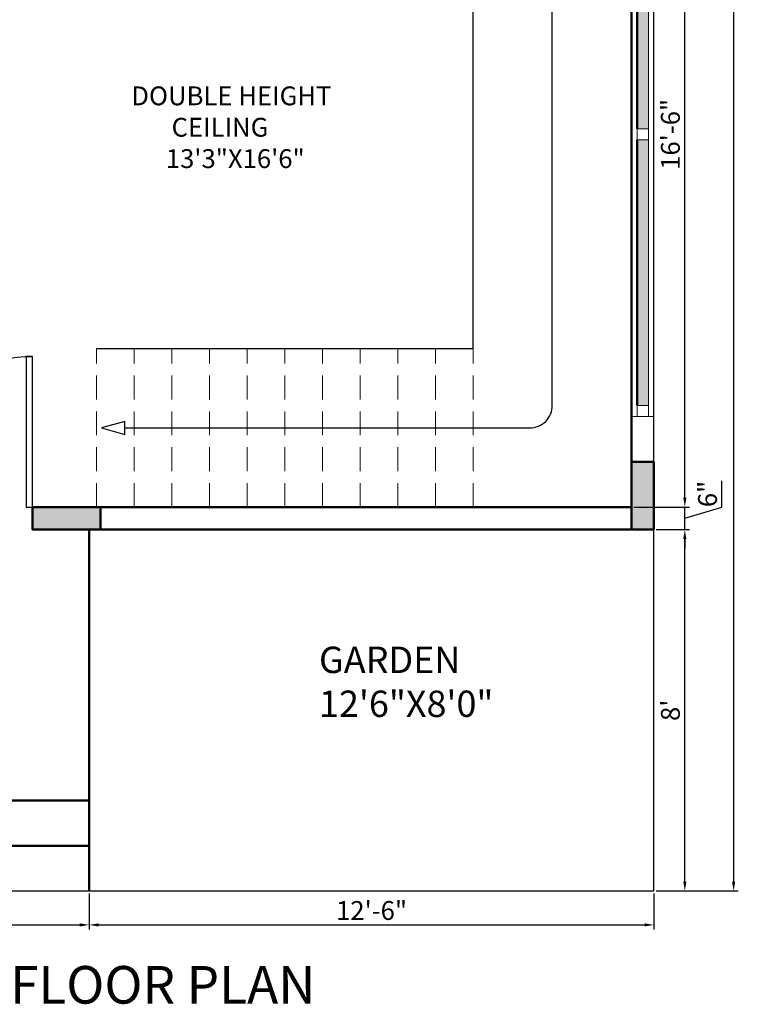
# Model space of a CAD drawing. Units: inches. Extents: x 3064 to 19385, y 846 to 15425.
# Tile 27 of 108: x 4938 to 5129, y 846 to 1108. Entities that reach past the tile are written whole.
import ezdxf

# ---------------------------------------------------------------- set-up
doc = ezdxf.new("R2010")
doc.units = ezdxf.units.IN
doc.linetypes.add('DASHED', pattern=[19.05, 12.7, -6.35])
for name, color, linetype, lineweight in [('A-ANNO-DIMS', 2, 'Continuous', 18), ('A-ANNO-TEXT', 7, 'Continuous', 25), ('A-AREA-IDEN', 3, 'Continuous', 18), ('A-COLS', 1, 'Continuous', 35), ('A-DOOR', 3, 'Continuous', 25), ('A-FLOR-STRS', 2, 'Continuous', 25), ('A-FLOR-STRS-OVHD', 2, 'DASHED', 18), ('A-GLAZ', 4, 'Continuous', 18), ('A-WALL', 7, 'Continuous', 50), ('C-PROP', 6, 'Continuous', 25)]:
    doc.layers.add(name, color=color, linetype=linetype, lineweight=lineweight)
doc.styles.get("Standard").update_dxf_attribs({"font": 'arial.ttf'})
doc.dimstyles.new('ISO-25', dxfattribs={"dimtxt": 9, "dimasz": 2.5, "dimexe": 1.25, "dimexo": 0.625, "dimtad": 1, "dimdec": 1, "dimlunit": 3, "dimtxsty": 'Standard', "dimcen": 2.5, "dimadec": 0, "dimazin": 0, "dimtfac": 1, "dimtdec": 1, "dimtmove": 0, "dimatfit": 3, "dimfxl": 1, "dimarcsym": 0})

# ---------------------------------------------------------------- blocks, each defined once
blk = doc.blocks.new('*U2')
for p, q in [((0, 0), (0, -6)), ((40, 0), (40, -6))]:
    blk.add_line(p, q)
blk.add_lwpolyline([(0, 0), (0, 40), (1.75, 40), (1.75, 0)], close=True)
blk.add_arc((0, 0), 40, 0, 90)
blk = doc.blocks.new('*D56')
at = {"layer": 'A-ANNO-DIMS', "color": 0, "lineweight": -2, "transparency": 16777216}
for p, q in [((4764.48, 875.47), (4764.48, 865.83)), ((4956.48, 875.47), (4956.48, 865.83)), ((4766.98, 867.08), (4953.98, 867.08))]:
    blk.add_line(p, q, dxfattribs=at)
at = {"layer": 'A-ANNO-DIMS', "color": 0, "transparency": 16777216}
for points in [[(4766.98, 867.5), (4766.98, 866.67), (4764.48, 867.08)], [(4953.98, 867.5), (4953.98, 866.67), (4956.48, 867.08)]]:
    blk.add_solid(points, dxfattribs=at)
at = {"layer": 'Defpoints', "color": 0, "transparency": 16777216}
for p in [(4764.48, 876.1), (4956.48, 876.1), (4956.48, 867.08)]:
    blk.add_point(p, dxfattribs=at)
at = {"layer": 'A-ANNO-DIMS', "color": 0, "transparency": 16777216, "insert": (4860.48, 870.26), "char_height": 5, "attachment_point": 5}
blk.add_mtext("16'", dxfattribs=at)
blk = doc.blocks.new('*D57')
at = {"layer": 'A-ANNO-DIMS', "color": 0, "lineweight": -2, "transparency": 16777216}
for p, q in [((4956.48, 875.47), (4956.48, 865.83)), ((5106.48, 875.47), (5106.48, 865.83)), ((4958.98, 867.08), (5103.98, 867.08))]:
    blk.add_line(p, q, dxfattribs=at)
at = {"layer": 'A-ANNO-DIMS', "color": 0, "transparency": 16777216}
for points in [[(4958.98, 867.5), (4958.98, 866.67), (4956.48, 867.08)], [(5103.98, 867.5), (5103.98, 866.67), (5106.48, 867.08)]]:
    blk.add_solid(points, dxfattribs=at)
at = {"layer": 'Defpoints', "color": 0, "transparency": 16777216}
for p in [(4956.48, 876.1), (5106.48, 876.1), (5106.48, 867.08)]:
    blk.add_point(p, dxfattribs=at)
at = {"layer": 'A-ANNO-DIMS', "color": 0, "transparency": 16777216, "insert": (5031.48, 870.26), "char_height": 5, "attachment_point": 5}
blk.add_mtext('12\'-6"', dxfattribs=at)
blk = doc.blocks.new('*D58')
at = {"layer": 'A-ANNO-DIMS', "color": 0, "lineweight": -2, "transparency": 16777216}
for p, q in [((5107.1, 972.1), (5115.92, 972.1)), ((5114.67, 878.6), (5114.67, 969.6)), ((5107.1, 876.1), (5115.92, 876.1))]:
    blk.add_line(p, q, dxfattribs=at)
at = {"layer": 'A-ANNO-DIMS', "color": 0, "transparency": 16777216}
for points in [[(5114.25, 969.6), (5115.09, 969.6), (5114.67, 972.1)], [(5114.25, 878.6), (5115.09, 878.6), (5114.67, 876.1)]]:
    blk.add_solid(points, dxfattribs=at)
at = {"layer": 'Defpoints', "color": 0, "transparency": 16777216}
for p in [(5106.48, 972.1), (5114.67, 972.1), (5106.48, 876.1)]:
    blk.add_point(p, dxfattribs=at)
at = {"layer": 'A-ANNO-DIMS', "color": 0, "transparency": 16777216, "insert": (5111.49, 924.1), "char_height": 5, "attachment_point": 5, "rotation": 90}
blk.add_mtext("8'", dxfattribs=at)
blk = doc.blocks.new('*D59')
at = {"layer": 'A-ANNO-DIMS', "color": 0, "lineweight": -2, "transparency": 16777216}
for p, q in [((5124.52, 978.05), (5124.52, 985.07)), ((5114.67, 980.6), (5114.67, 983.1)), ((5101.1, 978.1), (5115.92, 978.1)), ((5114.67, 972.1), (5114.67, 978.1)), ((5114.67, 972.1), (5114.67, 978.1)), ((5114.67, 975.1), (5124.52, 978.05)), ((5107.1, 972.1), (5115.92, 972.1)), ((5114.67, 969.6), (5114.67, 967.1))]:
    blk.add_line(p, q, dxfattribs=at)
at = {"layer": 'A-ANNO-DIMS', "color": 0, "transparency": 16777216}
for points in [[(5114.25, 980.6), (5115.09, 980.6), (5114.67, 978.1)], [(5114.25, 969.6), (5115.09, 969.6), (5114.67, 972.1)]]:
    blk.add_solid(points, dxfattribs=at)
at = {"layer": 'Defpoints', "color": 0, "transparency": 16777216}
for p in [(5100.48, 978.1), (5114.67, 978.1), (5106.48, 972.1)]:
    blk.add_point(p, dxfattribs=at)
at = {"layer": 'A-ANNO-DIMS', "color": 0, "transparency": 16777216, "insert": (5121.34, 981.56), "char_height": 5, "attachment_point": 5, "rotation": 90}
blk.add_mtext('6"', dxfattribs=at)
blk = doc.blocks.new('*D60')
at = {"layer": 'A-ANNO-DIMS', "color": 0, "lineweight": -2, "transparency": 16777216}
for p, q in [((5101.1, 1176.1), (5115.92, 1176.1)), ((5114.67, 980.6), (5114.67, 1173.6)), ((5101.1, 978.1), (5115.92, 978.1))]:
    blk.add_line(p, q, dxfattribs=at)
at = {"layer": 'A-ANNO-DIMS', "color": 0, "transparency": 16777216}
for points in [[(5114.25, 1173.6), (5115.09, 1173.6), (5114.67, 1176.1)], [(5114.25, 980.6), (5115.09, 980.6), (5114.67, 978.1)]]:
    blk.add_solid(points, dxfattribs=at)
at = {"layer": 'Defpoints', "color": 0, "transparency": 16777216}
for p in [(5100.48, 1176.1), (5114.67, 1176.1), (5100.48, 978.1)]:
    blk.add_point(p, dxfattribs=at)
at = {"layer": 'A-ANNO-DIMS', "color": 0, "transparency": 16777216, "insert": (5111.49, 1077.1), "char_height": 5, "attachment_point": 5, "rotation": 90}
blk.add_mtext('16\'-6"', dxfattribs=at)
blk = doc.blocks.new('*D66')
at = {"layer": 'A-ANNO-DIMS', "color": 0, "lineweight": -2, "transparency": 16777216}
for p, q in [((5107.1, 1392.1), (5128.87, 1392.1)), ((5127.62, 1389.6), (5127.62, 878.6)), ((5107.1, 876.1), (5128.87, 876.1))]:
    blk.add_line(p, q, dxfattribs=at)
at = {"layer": 'A-ANNO-DIMS', "color": 0, "transparency": 16777216}
for points in [[(5127.2, 1389.6), (5128.04, 1389.6), (5127.62, 1392.1)], [(5127.2, 878.6), (5128.04, 878.6), (5127.62, 876.1)]]:
    blk.add_solid(points, dxfattribs=at)
at = {"layer": 'Defpoints', "color": 0, "transparency": 16777216}
for p in [(5106.48, 1392.1), (5106.48, 876.1), (5127.62, 876.1)]:
    blk.add_point(p, dxfattribs=at)
at = {"layer": 'A-ANNO-DIMS', "color": 0, "transparency": 16777216, "insert": (5124.44, 1134.1), "char_height": 5, "attachment_point": 5, "rotation": 90}
blk.add_mtext("43'", dxfattribs=at)
blk = doc.blocks.new('WIN-1800-PAIR')
h = blk.add_hatch(color=256)
h.dxf.hatch_style = 1
h.paths.add_polyline_path([(0, 0), (3, 0), (3, 70.5), (0, 70.5)])
h.paths.add_polyline_path([(3, 144), (0, 144), (0, 73.5), (3, 73.5)])
blk.add_line((3, 144), (3, 73.5))
blk.add_lwpolyline([(3, 144), (0, 144), (0, 147), (3, 147)], close=True)
blk = doc.blocks.new('WIN-2000')
blk.add_line((3, 0), (3, 70.5))
blk.add_lwpolyline([(3, 70.5), (0, 70.5), (0, 73.5), (3, 73.5)], close=True)

msp = doc.modelspace()

# ---------------------------------------------------------------- hatches: boundary and pattern name
at = {"layer": 'A-COLS'}
h = msp.add_hatch(color=256, dxfattribs=at)
h.dxf.hatch_style = 1
h.paths.add_polyline_path([(5106.48, 972.1), (5106.48, 990.1), (5100.48, 990.1), (5100.48, 972.1)])
h = msp.add_hatch(color=256, dxfattribs=at)
h.dxf.hatch_style = 1
h.paths.add_polyline_path([(4959.48, 978.1), (4941.48, 978.1), (4941.48, 972.1), (4959.48, 972.1)])

# ---------------------------------------------------------------- linework, layer by layer
at = {"layer": 'A-FLOR-STRS'}
for q in [(5058.48, 1176.1), (4958.48, 1020.1)]:
    msp.add_line((5058.48, 1020.1), q, dxfattribs=at)
msp.add_lwpolyline([(4965.97, 999.1), (5073.48, 999.1, 0.414214), (5079.48, 1005.1), (5079.48, 1149.1, 0.414214), (5073.48, 1155.1), (4946.48, 1155.1)], format="xyb", dxfattribs=at)
msp.add_lwpolyline([(4959.77, 999.1), (4965.97, 997.36), (4965.97, 1000.83)], close=True, dxfattribs=at)
at = {"layer": 'A-FLOR-STRS-OVHD', "ltscale": 0.5}
for p, q in [((4958.48, 978.1), (4958.48, 1020.1)), ((4968.48, 978.1), (4968.48, 1020.1)), ((4978.48, 978.1), (4978.48, 1020.1)), ((4988.48, 978.1), (4988.48, 1020.1)), ((4998.48, 978.1), (4998.48, 1020.1)), ((5008.48, 978.1), (5008.48, 1020.1)), ((5018.48, 978.1), (5018.48, 1020.1)), ((5028.48, 978.1), (5028.48, 1020.1)), ((5038.48, 978.1), (5038.48, 1020.1)), ((5048.48, 978.1), (5048.48, 1020.1)), ((5058.48, 978.1), (5058.48, 1020.1))]:
    msp.add_line(p, q, dxfattribs=at)
at = {"layer": 'A-GLAZ'}
msp.add_line((5106.48, 1002.1), (5100.48, 1002.1), dxfattribs=at)
msp.add_line((5106.48, 1002.1), (5100.48, 1002.1), dxfattribs=at)
msp.add_lwpolyline([(5104.98, 1002.1), (5101.98, 1002.1), (5101.98, 1005.1), (5104.98, 1005.1)], close=True, dxfattribs=at)
at = {"layer": 'A-WALL'}
for p, q in [((5100.48, 978.1), (5100.48, 1176.1)), ((5101.98, 1149.1), (5101.98, 1078.6)), ((5101.98, 1005.1), (5101.98, 1075.6)), ((5100.48, 978.1), (4941.48, 978.1)), ((4941.48, 972.1), (4941.48, 978.1)), ((5106.48, 972.1), (4941.48, 972.1)), ((4956.48, 972.1), (4956.48, 876.1)), ((4764.48, 900.1), (4956.48, 900.1)), ((4764.48, 888.1), (4956.48, 888.1))]:
    msp.add_line(p, q, dxfattribs=at)
for points in [[(5106.48, 972.1), (5106.48, 990.1), (5100.48, 990.1), (5100.48, 972.1)], [(4959.48, 978.1), (4941.48, 978.1), (4941.48, 972.1), (4959.48, 972.1)]]:
    msp.add_lwpolyline(points, close=True, dxfattribs=at)
at = {"layer": 'C-PROP'}
for p, q in [((5106.48, 876.1), (5106.48, 1392.1)), ((4764.48, 876.1), (5106.48, 876.1))]:
    msp.add_line(p, q, dxfattribs=at)

# ---------------------------------------------------------------- block references
at = {"layer": 'A-DOOR', "xscale": -1}
msp.add_blockref('*U2', (4941.48, 978.1), dxfattribs=at)
at = {"layer": 'A-GLAZ'}
for name in ['WIN-1800-PAIR', 'WIN-2000']:
    msp.add_blockref(name, (5101.98, 1005.1), dxfattribs=at)

# ---------------------------------------------------------------- texts
at = {"layer": 'A-ANNO-TEXT', "insert": (4875.14, 856.17), "char_height": 10, "attachment_point": 1}
msp.add_mtext_dynamic_manual_height_columns('GROUND FLOOR PLAN', width=200.9739, gutter_width=12.5, heights=[0], dxfattribs=at)
at = {"layer": 'A-AREA-IDEN', "attachment_point": 1}
for s, width, insert, char_height in [('DOUBLE HEIGHT \\P       CEILING            \\P      13\'3"X16\'6"', 57.0817, (4967.68, 1089.82), 5), ('GARDEN\\P12\'6"X8\'0"', 67.5924, (5017.52, 941), 7)]:
    msp.add_mtext_dynamic_manual_height_columns(s, width=width, gutter_width=12.5, heights=[0], dxfattribs=dict(at, insert=insert, char_height=char_height))

# ---------------------------------------------------------------- dimensions: what is measured, and where the dimension line sits
at = {"layer": 'A-ANNO-DIMS'}
for base, p1, p2, override, picture, middle in [((5127.62, 876.1), (5106.48, 1392.1), (5106.48, 876.1), {"dimtxt": 5, "dimclrd": 0, "dimclre": 0, "dimclrt": 0}, '*D66', (5124.44, 1134.1)), ((5114.67, 1176.1), (5100.48, 978.1), (5100.48, 1176.1), {"dimtxt": 5, "dimclrd": 0, "dimclre": 0, "dimclrt": 0, "dimtmove": 1}, '*D60', (5111.49, 1077.1)), ((5114.67, 978.1), (5106.48, 972.1), (5100.48, 978.1), {"dimtxt": 5, "dimclrd": 0, "dimclre": 0, "dimclrt": 0, "dimtmove": 1}, '*D59', (5121.34, 978.68)), ((5114.67, 972.1), (5106.48, 876.1), (5106.48, 972.1), {"dimtxt": 5, "dimclrd": 0, "dimclre": 0, "dimclrt": 0}, '*D58', (5111.49, 924.1))]:
    dim = msp.add_linear_dim(base=base, p1=p1, p2=p2, angle=90, dimstyle='ISO-25', override=override, dxfattribs=at)
    dim.commit()
    dim.dimension.update_dxf_attribs({"geometry": picture, "text_midpoint": middle})
for base, p1, p2, override, picture, middle in [((4956.48, 867.08), (4764.48, 876.1), (4956.48, 876.1), {"dimtxt": 5, "dimclrd": 0, "dimclre": 0, "dimclrt": 0}, '*D56', (4860.48, 870.26)), ((5106.48, 867.08), (4956.48, 876.1), (5106.48, 876.1), {"dimtxt": 5, "dimclrd": 0, "dimclre": 0, "dimclrt": 0, "dimtmove": 1}, '*D57', (5031.48, 870.26))]:
    dim = msp.add_linear_dim(base=base, p1=p1, p2=p2, dimstyle='ISO-25', override=override, dxfattribs=at)
    dim.commit()
    dim.dimension.update_dxf_attribs({"geometry": picture, "text_midpoint": middle})

doc.saveas('drawing.dxf')
